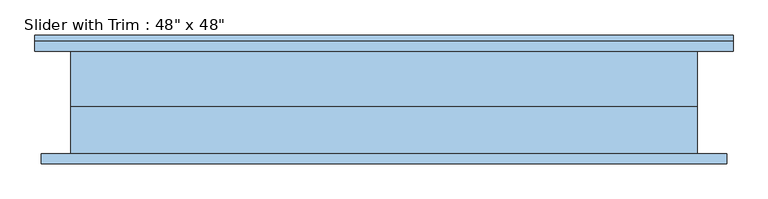
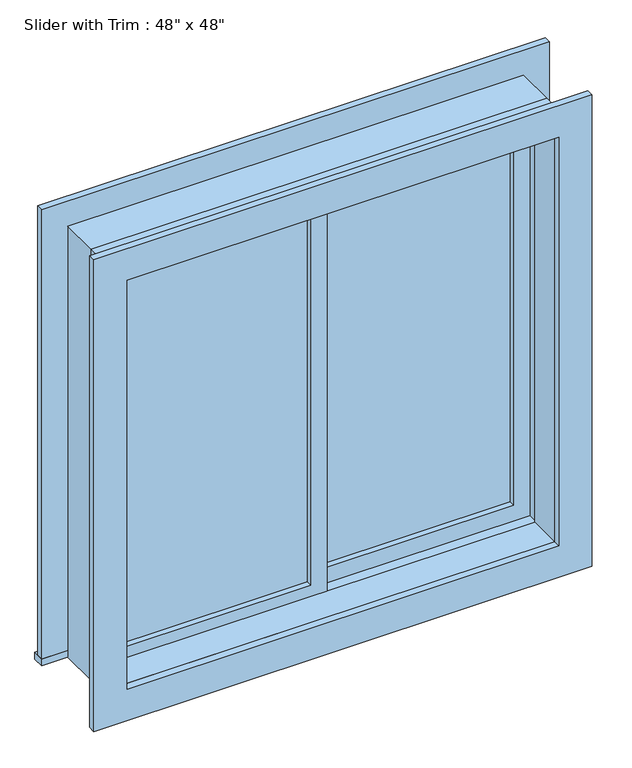
"""IFC4 building model written with IfcOpenShell, lengths in millimetres: window geometry."""

from ifc_helpers import new_model, si_unit, frame, origin, place, context, project, spatial, polyline, outline, extrude, source, transform, mapped, element, save


def window_deda82dd(model_context):
    return source(origin(), model_context, "Body", "SweptSolid", [
        extrude(outline(polyline([(-546.1, 20.625), (-22.225, 20.625), (-22.225, 7.925), (-546.1, 7.925), (-546.1, 20.625)])), frame((0.0, 0.0, 977.9), z_axis=(0.0, 0.0, 1.0), x_axis=(1.0, 0.0, 0.0)), (0.0, 0.0, 1.0), 1092.2),
        extrude(outline(polyline([(2114.55, -590.55), (933.45, -590.55), (933.45, 22.225), (2114.55, 22.225), (2114.55, -590.55)]), holes=[polyline([(2070.1, -546.1), (2070.1, -22.225), (977.9, -22.225), (977.9, -546.1), (2070.1, -546.1)])]), frame((0.0, -7.95, 0.0), z_axis=(0.0, 1.0, 0.0), x_axis=(0.0, 0.0, 1.0)), (0.0, 0.0, 1.0), 44.45),
        extrude(outline(polyline([(-679.45, 131.75), (679.45, 131.75), (679.45, 100.0), (-679.45, 100.0), (-679.45, 131.75)])), frame((0.0, 0.0, 914.4), z_axis=(0.0, 0.0, 1.0), x_axis=(1.0, 0.0, 0.0)), (0.0, 0.0, 1.0), 19.05),
        extrude(outline(polyline([(2114.55, -590.55), (2114.55, 590.55), (933.45, 590.55), (933.45, 679.45), (2203.45, 679.45), (2203.45, -679.45), (933.45, -679.45), (933.45, -590.55), (2114.55, -590.55)])), frame((0.0, 100.0, 0.0), z_axis=(0.0, 1.0, 0.0), x_axis=(0.0, 0.0, 1.0)), (0.0, 0.0, 1.0), 19.05),
        extrude(outline(polyline([(2190.75, 666.75), (2190.75, -666.75), (857.25, -666.75), (857.25, 666.75), (2190.75, 666.75)]), holes=[polyline([(2101.85, 577.85), (946.15, 577.85), (946.15, -577.85), (2101.85, -577.85), (2101.85, 577.85)])]), frame((0.0, -119.05, 0.0), z_axis=(0.0, 1.0, 0.0), x_axis=(0.0, 0.0, 1.0)), (0.0, 0.0, 1.0), 19.05),
        extrude(outline(polyline([(546.1, 52.375), (22.225, 52.375), (22.225, 65.075), (546.1, 65.075), (546.1, 52.375)])), frame((0.0, 0.0, 977.9), z_axis=(0.0, 0.0, 1.0), x_axis=(1.0, 0.0, 0.0)), (0.0, 0.0, 1.0), 1092.2),
        extrude(outline(polyline([(2114.55, -22.225), (933.45, -22.225), (933.45, 590.55), (2114.55, 590.55), (2114.55, -22.225)]), holes=[polyline([(2070.1, 22.225), (2070.1, 546.1), (977.9, 546.1), (977.9, 22.225), (2070.1, 22.225)])]), frame((0.0, 36.5, 0.0), z_axis=(0.0, 1.0, 0.0), x_axis=(0.0, 0.0, 1.0)), (0.0, 0.0, 1.0), 44.45),
        extrude(outline(polyline([(2133.6, -609.6), (914.4, -609.6), (914.4, 609.6), (2133.6, 609.6), (2133.6, -609.6)]), holes=[polyline([(2101.85, -577.85), (2101.85, 577.85), (946.15, 577.85), (946.15, -577.85), (2101.85, -577.85)])]), frame((0.0, -100.0, 0.0), z_axis=(0.0, 1.0, 0.0), x_axis=(0.0, 0.0, 1.0)), (0.0, 0.0, 1.0), 92.05),
        extrude(outline(polyline([(2133.6, 609.6), (2133.6, -609.6), (914.4, -609.6), (914.4, 609.6), (2133.6, 609.6)]), holes=[polyline([(2114.55, 590.55), (933.45, 590.55), (933.45, -590.55), (2114.55, -590.55), (2114.55, 590.55)])]), frame((0.0, -7.95, 0.0), z_axis=(0.0, 1.0, 0.0), x_axis=(0.0, 0.0, 1.0)), (0.0, 0.0, 1.0), 107.95),
    ])


if __name__ == "__main__":
    model = new_model("IFC4")
    model_context = context("Model", 3, world=origin())
    ifc_project = project(units=[si_unit("LENGTHUNIT", "METRE", prefix="MILLI")], contexts=[model_context])
    site = spatial("IfcSite", under=ifc_project)
    building = spatial("IfcBuilding", under=site)
    placement = place(None, origin())
    window_shape = window_deda82dd(model_context)
    element("IfcWindow", 1, ObjectType="Slider with Trim : 48\" x 48\"", at=placement, inside=building, context=model_context, shape_type="MappedRepresentation", body=[
        mapped(window_shape, transform((0.0, 0.0, 0.0), x_axis=(1.0, 0.0, 0.0), y_axis=(0.0, 1.0, 0.0), z_axis=(0.0, 0.0, 1.0))),
    ])
    save(model, "model.ifc")

# Revit data of these elements
# Type "Slider with Trim : 48\" x 48\""
#   Type Mark = "24"
#   Construction Type Id = "GSP4R"
#   Assembly Code = "B2020100"
#   Analytic Construction = "1/8 in Pilkington single glazing"
#   Visual Light Transmittance = 0.9
#   Solar Heat Gain Coefficient = 0.78
#   Heat Transfer Coefficient (U) = 3.6886 W/(m²·K)
#   Height = 4' - 0"
#   Default Sill Height = 3' - 0"
#   Trim Projection - Ext. = 0' - 0 3/4"
#   Trim Projection - Int. = 0' - 0 3/4"
#   Trim Width - Exterior = 0' - 3 1/2"
#   Trim Width - Interior = 0' - 3 1/2"
#   Width = 4' - 0"
#   Window Inset = 0' - 0 3/4"
#   Define Thermal Properties by = 1
#   Glass Pane Material = Glass
#   Sash Material = Sash
#   Trim Exterior Material = Trim
#   Trim Interior Material = Trim
#   Wall Closure = (empty or 0)
# Element 1 (IfcWindow, "Slider with Trim : 48\" x 48\"")
#   Materials on its faces: "Sash", "Trim", "Glass"
# Materials
#   "Glass": class "Glass", colour RGB 218 227 224, transparency 0.85, Description = "Soda Lime Glass", Cost = 0
#   "Sash": class "Wood", colour RGB 136 99 55, transparency 0
#   "Trim": class "Wood", colour RGB 224 178 126, transparency 0
